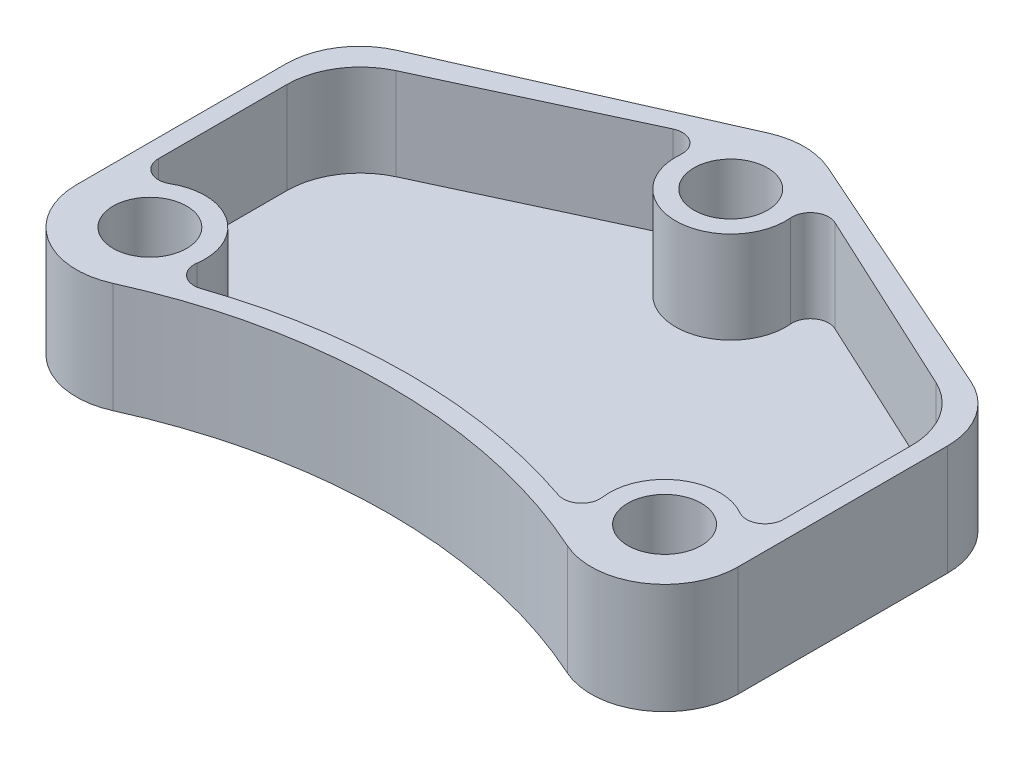
ISO-10303-21;
HEADER;
FILE_DESCRIPTION(('STEP AP214'),'2;1');
FILE_NAME('part.step','',(''),(''),'','','');
FILE_SCHEMA(('AUTOMOTIVE_DESIGN { 1 0 10303 214 1 1 1 1 }'));
ENDSEC;
DATA;
#1=APPLICATION_CONTEXT('core data for automotive mechanical design processes');
#2=APPLICATION_PROTOCOL_DEFINITION('international standard','automotive_design',2000,#1);
#3=PRODUCT_CONTEXT('',#1,'mechanical');
#4=PRODUCT('Part','Part','',(#3));
#5=PRODUCT_RELATED_PRODUCT_CATEGORY('part','',(#4));
#6=PRODUCT_DEFINITION_FORMATION('','',#4);
#7=PRODUCT_DEFINITION_CONTEXT('part definition',#1,'design');
#8=PRODUCT_DEFINITION('design','',#6,#7);
#9=PRODUCT_DEFINITION_SHAPE('','',#8);
#10=(LENGTH_UNIT() NAMED_UNIT(*) SI_UNIT(.MILLI.,.METRE.));
#11=(NAMED_UNIT(*) PLANE_ANGLE_UNIT() SI_UNIT($,.RADIAN.));
#12=(NAMED_UNIT(*) SI_UNIT($,.STERADIAN.) SOLID_ANGLE_UNIT());
#13=UNCERTAINTY_MEASURE_WITH_UNIT(LENGTH_MEASURE(1.E-05),#10,'distance_accuracy_value','');
#14=(GEOMETRIC_REPRESENTATION_CONTEXT(3) GLOBAL_UNCERTAINTY_ASSIGNED_CONTEXT((#13)) GLOBAL_UNIT_ASSIGNED_CONTEXT((#10,
#11,#12)) REPRESENTATION_CONTEXT('',''));
#15=CARTESIAN_POINT('',(0.,0.,0.));
#16=DIRECTION('',(0.,0.,1.));
#17=DIRECTION('',(1.,0.,0.));
#18=AXIS2_PLACEMENT_3D('',#15,#16,#17);
#19=CARTESIAN_POINT('',(70.,30.,88.0000000000001));
#20=DIRECTION('',(0.,-1.,0.));
#21=DIRECTION('',(0.,0.,-1.));
#22=AXIS2_PLACEMENT_3D('',#19,#20,#21);
#23=CYLINDRICAL_SURFACE('',#22,15.);
#24=DIRECTION('',(0.,-1.,0.));
#25=VECTOR('',#24,1.);
#26=CARTESIAN_POINT('',(77.5,30.,75.0096189432336));
#27=LINE('',#26,#25);
#28=CARTESIAN_POINT('',(77.5,30.,75.0096189432336));
#29=VERTEX_POINT('',#28);
#30=CARTESIAN_POINT('',(77.5,5.,75.0096189432336));
#31=VERTEX_POINT('',#30);
#32=EDGE_CURVE('E62',#29,#31,#27,.T.);
#33=ORIENTED_EDGE('',*,*,#32,.T.);
#34=CARTESIAN_POINT('',(70.,5.,88.0000000000001));
#35=DIRECTION('',(0.,-1.,0.));
#36=DIRECTION('',(0.,0.,-1.));
#37=AXIS2_PLACEMENT_3D('',#34,#35,#36);
#38=CIRCLE('',#37,15.);
#39=CARTESIAN_POINT('',(55.1442718779015,5.,90.0754136846162));
#40=VERTEX_POINT('',#39);
#41=EDGE_CURVE('E57',#31,#40,#38,.F.);
#42=ORIENTED_EDGE('',*,*,#41,.T.);
#43=DIRECTION('',(0.,-1.,0.));
#44=VECTOR('',#43,1.);
#45=CARTESIAN_POINT('',(55.1442718779015,30.,90.0754136846162));
#46=LINE('',#45,#44);
#47=CARTESIAN_POINT('',(55.1442718779015,30.,90.0754136846162));
#48=VERTEX_POINT('',#47);
#49=EDGE_CURVE('E47',#48,#40,#46,.T.);
#50=ORIENTED_EDGE('',*,*,#49,.F.);
#51=CARTESIAN_POINT('',(70.,30.,88.0000000000001));
#52=DIRECTION('',(0.,1.,0.));
#53=DIRECTION('',(0.,0.,1.));
#54=AXIS2_PLACEMENT_3D('',#51,#52,#53);
#55=CIRCLE('',#54,15.);
#56=EDGE_CURVE('E343',#48,#29,#55,.F.);
#57=ORIENTED_EDGE('',*,*,#56,.T.);
#58=EDGE_LOOP('',(#33,#42,#50,#57));
#59=FACE_BOUND('',#58,.T.);
#60=ADVANCED_FACE('F41',(#59),#23,.T.);
#61=CARTESIAN_POINT('',(50.1923625038687,30.,90.7672182461548));
#62=DIRECTION('',(0.,-1.,0.));
#63=DIRECTION('',(0.,0.,-1.));
#64=AXIS2_PLACEMENT_3D('',#61,#62,#63);
#65=CYLINDRICAL_SURFACE('',#64,4.99999999999999);
#66=CARTESIAN_POINT('',(50.1923625038687,5.,90.7672182461548));
#67=DIRECTION('',(0.,-1.,0.));
#68=DIRECTION('',(0.,0.,-1.));
#69=AXIS2_PLACEMENT_3D('',#66,#67,#68);
#70=CIRCLE('',#69,4.99999999999999);
#71=CARTESIAN_POINT('',(48.5732540360019,5.,95.497808882564));
#72=VERTEX_POINT('',#71);
#73=EDGE_CURVE('E378',#72,#40,#70,.F.);
#74=ORIENTED_EDGE('',*,*,#73,.F.);
#75=DIRECTION('',(0.,-1.,0.));
#76=VECTOR('',#75,1.);
#77=CARTESIAN_POINT('',(48.5732540360019,30.,95.497808882564));
#78=LINE('',#77,#76);
#79=CARTESIAN_POINT('',(48.5732540360019,30.,95.497808882564));
#80=VERTEX_POINT('',#79);
#81=EDGE_CURVE('E247',#80,#72,#78,.T.);
#82=ORIENTED_EDGE('',*,*,#81,.F.);
#83=CARTESIAN_POINT('',(50.1923625038687,30.,90.7672182461548));
#84=DIRECTION('',(0.,1.,0.));
#85=DIRECTION('',(0.,0.,1.));
#86=AXIS2_PLACEMENT_3D('',#83,#84,#85);
#87=CIRCLE('',#86,4.99999999999999);
#88=EDGE_CURVE('E345',#48,#80,#87,.F.);
#89=ORIENTED_EDGE('',*,*,#88,.F.);
#90=ORIENTED_EDGE('',*,*,#49,.T.);
#91=EDGE_LOOP('',(#74,#82,#89,#90));
#92=FACE_BOUND('',#91,.T.);
#93=ADVANCED_FACE('F428',(#92),#65,.F.);
#94=CARTESIAN_POINT('',(0.,30.,237.415527974839));
#95=DIRECTION('',(0.,-1.,0.));
#96=DIRECTION('',(0.,0.,-1.));
#97=AXIS2_PLACEMENT_3D('',#94,#95,#96);
#98=CYLINDRICAL_SURFACE('',#97,150.);
#99=ORIENTED_EDGE('',*,*,#81,.T.);
#100=CARTESIAN_POINT('',(0.,5.,237.415527974839));
#101=DIRECTION('',(0.,-1.,0.));
#102=DIRECTION('',(0.,0.,-1.));
#103=AXIS2_PLACEMENT_3D('',#100,#101,#102);
#104=CIRCLE('',#103,150.);
#105=CARTESIAN_POINT('',(-48.573254036002,5.,95.497808882564));
#106=VERTEX_POINT('',#105);
#107=EDGE_CURVE('E379',#72,#106,#104,.F.);
#108=ORIENTED_EDGE('',*,*,#107,.T.);
#109=DIRECTION('',(0.,-1.,0.));
#110=VECTOR('',#109,1.);
#111=CARTESIAN_POINT('',(-48.573254036002,30.,95.497808882564));
#112=LINE('',#111,#110);
#113=CARTESIAN_POINT('',(-48.573254036002,30.,95.497808882564));
#114=VERTEX_POINT('',#113);
#115=EDGE_CURVE('E244',#114,#106,#112,.T.);
#116=ORIENTED_EDGE('',*,*,#115,.F.);
#117=CARTESIAN_POINT('',(0.,30.,237.415527974839));
#118=DIRECTION('',(0.,1.,0.));
#119=DIRECTION('',(0.,0.,1.));
#120=AXIS2_PLACEMENT_3D('',#117,#118,#119);
#121=CIRCLE('',#120,150.);
#122=EDGE_CURVE('E338',#114,#80,#121,.F.);
#123=ORIENTED_EDGE('',*,*,#122,.T.);
#124=EDGE_LOOP('',(#99,#108,#116,#123));
#125=FACE_BOUND('',#124,.T.);
#126=ADVANCED_FACE('F431',(#125),#98,.T.);
#127=CARTESIAN_POINT('',(-50.1923625038687,30.,90.7672182461548));
#128=DIRECTION('',(0.,-1.,0.));
#129=DIRECTION('',(0.,0.,-1.));
#130=AXIS2_PLACEMENT_3D('',#127,#128,#129);
#131=CYLINDRICAL_SURFACE('',#130,4.99999999999999);
#132=ORIENTED_EDGE('',*,*,#115,.T.);
#133=CARTESIAN_POINT('',(-50.1923625038687,5.,90.7672182461548));
#134=DIRECTION('',(0.,-1.,0.));
#135=DIRECTION('',(0.,0.,-1.));
#136=AXIS2_PLACEMENT_3D('',#133,#134,#135);
#137=CIRCLE('',#136,4.99999999999999);
#138=CARTESIAN_POINT('',(-55.1442718779016,5.,90.0754136846162));
#139=VERTEX_POINT('',#138);
#140=EDGE_CURVE('E382',#106,#139,#137,.T.);
#141=ORIENTED_EDGE('',*,*,#140,.T.);
#142=DIRECTION('',(0.,-1.,0.));
#143=VECTOR('',#142,1.);
#144=CARTESIAN_POINT('',(-55.1442718779016,30.,90.0754136846162));
#145=LINE('',#144,#143);
#146=CARTESIAN_POINT('',(-55.1442718779016,30.,90.0754136846162));
#147=VERTEX_POINT('',#146);
#148=EDGE_CURVE('E245',#147,#139,#145,.T.);
#149=ORIENTED_EDGE('',*,*,#148,.F.);
#150=CARTESIAN_POINT('',(-50.1923625038687,30.,90.7672182461548));
#151=DIRECTION('',(0.,1.,0.));
#152=DIRECTION('',(0.,0.,1.));
#153=AXIS2_PLACEMENT_3D('',#150,#151,#152);
#154=CIRCLE('',#153,4.99999999999999);
#155=EDGE_CURVE('E336',#147,#114,#154,.T.);
#156=ORIENTED_EDGE('',*,*,#155,.T.);
#157=EDGE_LOOP('',(#132,#141,#149,#156));
#158=FACE_BOUND('',#157,.T.);
#159=ADVANCED_FACE('F432',(#158),#131,.F.);
#160=CARTESIAN_POINT('',(-70.,30.,88.0000000000001));
#161=DIRECTION('',(0.,-1.,0.));
#162=DIRECTION('',(0.,0.,-1.));
#163=AXIS2_PLACEMENT_3D('',#160,#161,#162);
#164=CYLINDRICAL_SURFACE('',#163,15.);
#165=CARTESIAN_POINT('',(-70.,5.,88.0000000000001));
#166=DIRECTION('',(0.,-1.,0.));
#167=DIRECTION('',(0.,0.,-1.));
#168=AXIS2_PLACEMENT_3D('',#165,#166,#167);
#169=CIRCLE('',#168,15.);
#170=CARTESIAN_POINT('',(-77.5,5.,75.0096189432336));
#171=VERTEX_POINT('',#170);
#172=EDGE_CURVE('E387',#171,#139,#169,.T.);
#173=ORIENTED_EDGE('',*,*,#172,.F.);
#174=DIRECTION('',(0.,-1.,0.));
#175=VECTOR('',#174,1.);
#176=CARTESIAN_POINT('',(-77.5000000000001,30.,75.0096189432335));
#177=LINE('',#176,#175);
#178=CARTESIAN_POINT('',(-77.5000000000001,30.,75.0096189432335));
#179=VERTEX_POINT('',#178);
#180=EDGE_CURVE('E239',#179,#171,#177,.T.);
#181=ORIENTED_EDGE('',*,*,#180,.F.);
#182=CARTESIAN_POINT('',(-70.,30.,88.0000000000001));
#183=DIRECTION('',(0.,1.,0.));
#184=DIRECTION('',(0.,0.,1.));
#185=AXIS2_PLACEMENT_3D('',#182,#183,#184);
#186=CIRCLE('',#185,15.);
#187=EDGE_CURVE('E334',#147,#179,#186,.T.);
#188=ORIENTED_EDGE('',*,*,#187,.F.);
#189=ORIENTED_EDGE('',*,*,#148,.T.);
#190=EDGE_LOOP('',(#173,#181,#188,#189));
#191=FACE_BOUND('',#190,.T.);
#192=ADVANCED_FACE('F445',(#191),#164,.T.);
#193=CARTESIAN_POINT('',(-80.0000000000001,30.,70.6794919243114));
#194=DIRECTION('',(0.,-1.,0.));
#195=DIRECTION('',(0.,0.,-1.));
#196=AXIS2_PLACEMENT_3D('',#193,#194,#195);
#197=CYLINDRICAL_SURFACE('',#196,5.00000000000001);
#198=CARTESIAN_POINT('',(-80.0000000000001,5.,70.6794919243114));
#199=DIRECTION('',(0.,-1.,0.));
#200=DIRECTION('',(0.,0.,-1.));
#201=AXIS2_PLACEMENT_3D('',#198,#199,#200);
#202=CIRCLE('',#201,5.00000000000001);
#203=CARTESIAN_POINT('',(-85.0000000000001,5.,70.6794919243114));
#204=VERTEX_POINT('',#203);
#205=EDGE_CURVE('E386',#204,#171,#202,.F.);
#206=ORIENTED_EDGE('',*,*,#205,.F.);
#207=DIRECTION('',(0.,-1.,0.));
#208=VECTOR('',#207,1.);
#209=CARTESIAN_POINT('',(-85.0000000000001,30.,70.6794919243114));
#210=LINE('',#209,#208);
#211=CARTESIAN_POINT('',(-85.0000000000001,30.,70.6794919243114));
#212=VERTEX_POINT('',#211);
#213=EDGE_CURVE('E237',#212,#204,#210,.T.);
#214=ORIENTED_EDGE('',*,*,#213,.F.);
#215=CARTESIAN_POINT('',(-80.0000000000001,30.,70.6794919243114));
#216=DIRECTION('',(0.,1.,0.));
#217=DIRECTION('',(0.,0.,1.));
#218=AXIS2_PLACEMENT_3D('',#215,#216,#217);
#219=CIRCLE('',#218,5.00000000000001);
#220=EDGE_CURVE('E332',#179,#212,#219,.F.);
#221=ORIENTED_EDGE('',*,*,#220,.F.);
#222=ORIENTED_EDGE('',*,*,#180,.T.);
#223=EDGE_LOOP('',(#206,#214,#221,#222));
#224=FACE_BOUND('',#223,.T.);
#225=ADVANCED_FACE('F447',(#224),#197,.F.);
#226=CARTESIAN_POINT('',(-85.,30.,0.));
#227=DIRECTION('',(1.,0.,0.));
#228=DIRECTION('',(0.,0.,-1.));
#229=AXIS2_PLACEMENT_3D('',#226,#227,#228);
#230=PLANE('',#229);
#231=ORIENTED_EDGE('',*,*,#213,.T.);
#232=DIRECTION('',(0.,0.,-1.));
#233=VECTOR('',#232,1.);
#234=CARTESIAN_POINT('',(-85.,5.,0.));
#235=LINE('',#234,#233);
#236=CARTESIAN_POINT('',(-85.0000000000001,5.,35.7709926715189));
#237=VERTEX_POINT('',#236);
#238=EDGE_CURVE('E395',#204,#237,#235,.T.);
#239=ORIENTED_EDGE('',*,*,#238,.T.);
#240=DIRECTION('',(0.,-1.,0.));
#241=VECTOR('',#240,1.);
#242=CARTESIAN_POINT('',(-85.0000000000001,30.,35.7709926715189));
#243=LINE('',#242,#241);
#244=CARTESIAN_POINT('',(-85.0000000000001,30.,35.7709926715189));
#245=VERTEX_POINT('',#244);
#246=EDGE_CURVE('E232',#245,#237,#243,.T.);
#247=ORIENTED_EDGE('',*,*,#246,.F.);
#248=DIRECTION('',(0.,0.,1.));
#249=VECTOR('',#248,1.);
#250=CARTESIAN_POINT('',(-85.,30.,0.));
#251=LINE('',#250,#249);
#252=EDGE_CURVE('E327',#245,#212,#251,.T.);
#253=ORIENTED_EDGE('',*,*,#252,.T.);
#254=EDGE_LOOP('',(#231,#239,#247,#253));
#255=FACE_BOUND('',#254,.T.);
#256=ADVANCED_FACE('F451',(#255),#230,.T.);
#257=CARTESIAN_POINT('',(-65.0000000000001,30.,35.7709926715189));
#258=DIRECTION('',(0.,-1.,0.));
#259=DIRECTION('',(0.,0.,-1.));
#260=AXIS2_PLACEMENT_3D('',#257,#258,#259);
#261=CYLINDRICAL_SURFACE('',#260,20.);
#262=ORIENTED_EDGE('',*,*,#246,.T.);
#263=CARTESIAN_POINT('',(-65.0000000000001,5.,35.7709926715189));
#264=DIRECTION('',(0.,-1.,0.));
#265=DIRECTION('',(0.,0.,-1.));
#266=AXIS2_PLACEMENT_3D('',#263,#264,#265);
#267=CIRCLE('',#266,20.);
#268=CARTESIAN_POINT('',(-73.4399590477228,5.,17.639056997886));
#269=VERTEX_POINT('',#268);
#270=EDGE_CURVE('E394',#237,#269,#267,.T.);
#271=ORIENTED_EDGE('',*,*,#270,.T.);
#272=DIRECTION('',(0.,-1.,0.));
#273=VECTOR('',#272,1.);
#274=CARTESIAN_POINT('',(-73.4399590477228,30.,17.639056997886));
#275=LINE('',#274,#273);
#276=CARTESIAN_POINT('',(-73.4399590477228,30.,17.639056997886));
#277=VERTEX_POINT('',#276);
#278=EDGE_CURVE('E229',#277,#269,#275,.T.);
#279=ORIENTED_EDGE('',*,*,#278,.F.);
#280=CARTESIAN_POINT('',(-65.0000000000001,30.,35.7709926715189));
#281=DIRECTION('',(0.,1.,0.));
#282=DIRECTION('',(0.,0.,1.));
#283=AXIS2_PLACEMENT_3D('',#280,#281,#282);
#284=CIRCLE('',#283,20.);
#285=EDGE_CURVE('E324',#277,#245,#284,.T.);
#286=ORIENTED_EDGE('',*,*,#285,.T.);
#287=EDGE_LOOP('',(#262,#271,#279,#286));
#288=FACE_BOUND('',#287,.T.);
#289=ADVANCED_FACE('F454',(#288),#261,.F.);
#290=CARTESIAN_POINT('',(-6.32996928579205,30.,-13.5989517552247));
#291=DIRECTION('',(-0.421997952386136,0.,-0.906596783681648));
#292=DIRECTION('',(-0.906596783681648,0.,0.421997952386136));
#293=AXIS2_PLACEMENT_3D('',#290,#291,#292);
#294=PLANE('',#293);
#295=DIRECTION('',(-0.906596783681648,0.,0.421997952386136));
#296=VECTOR('',#295,1.);
#297=CARTESIAN_POINT('',(-6.32996928579205,5.,-13.5989517552247));
#298=LINE('',#297,#296);
#299=CARTESIAN_POINT('',(-22.0326861989435,5.,-6.28973281299653));
#300=VERTEX_POINT('',#299);
#301=EDGE_CURVE('E397',#300,#269,#298,.T.);
#302=ORIENTED_EDGE('',*,*,#301,.F.);
#303=DIRECTION('',(0.,-1.,0.));
#304=VECTOR('',#303,1.);
#305=CARTESIAN_POINT('',(-22.0326861989435,30.,-6.28973281299653));
#306=LINE('',#305,#304);
#307=CARTESIAN_POINT('',(-22.0326861989435,30.,-6.28973281299653));
#308=VERTEX_POINT('',#307);
#309=EDGE_CURVE('E230',#308,#300,#306,.T.);
#310=ORIENTED_EDGE('',*,*,#309,.F.);
#311=DIRECTION('',(0.906596783681648,0.,-0.421997952386136));
#312=VECTOR('',#311,1.);
#313=CARTESIAN_POINT('',(-6.32996928579205,30.,-13.5989517552247));
#314=LINE('',#313,#312);
#315=EDGE_CURVE('E325',#277,#308,#314,.T.);
#316=ORIENTED_EDGE('',*,*,#315,.F.);
#317=ORIENTED_EDGE('',*,*,#278,.T.);
#318=EDGE_LOOP('',(#302,#310,#316,#317));
#319=FACE_BOUND('',#318,.T.);
#320=ADVANCED_FACE('F722',(#319),#294,.F.);
#321=CARTESIAN_POINT('',(-19.9226964370129,30.,-1.75674889458829));
#322=DIRECTION('',(0.,-1.,0.));
#323=DIRECTION('',(0.,0.,-1.));
#324=AXIS2_PLACEMENT_3D('',#321,#322,#323);
#325=CYLINDRICAL_SURFACE('',#324,5.);
#326=CARTESIAN_POINT('',(-19.9226964370129,5.,-1.75674889458829));
#327=DIRECTION('',(0.,-1.,0.));
#328=DIRECTION('',(0.,0.,-1.));
#329=AXIS2_PLACEMENT_3D('',#326,#327,#328);
#330=CIRCLE('',#329,5.);
#331=CARTESIAN_POINT('',(-14.9420223277596,5.,-1.31756167094121));
#332=VERTEX_POINT('',#331);
#333=EDGE_CURVE('E402',#332,#300,#330,.F.);
#334=ORIENTED_EDGE('',*,*,#333,.F.);
#335=DIRECTION('',(0.,-1.,0.));
#336=VECTOR('',#335,1.);
#337=CARTESIAN_POINT('',(-14.9420223277596,30.,-1.31756167094121));
#338=LINE('',#337,#336);
#339=CARTESIAN_POINT('',(-14.9420223277596,30.,-1.31756167094121));
#340=VERTEX_POINT('',#339);
#341=EDGE_CURVE('E221',#340,#332,#338,.T.);
#342=ORIENTED_EDGE('',*,*,#341,.F.);
#343=CARTESIAN_POINT('',(-19.9226964370129,30.,-1.75674889458829));
#344=DIRECTION('',(0.,1.,0.));
#345=DIRECTION('',(0.,0.,1.));
#346=AXIS2_PLACEMENT_3D('',#343,#344,#345);
#347=CIRCLE('',#346,5.);
#348=EDGE_CURVE('E317',#308,#340,#347,.F.);
#349=ORIENTED_EDGE('',*,*,#348,.F.);
#350=ORIENTED_EDGE('',*,*,#309,.T.);
#351=EDGE_LOOP('',(#334,#342,#349,#350));
#352=FACE_BOUND('',#351,.T.);
#353=ADVANCED_FACE('F713',(#352),#325,.F.);
#354=CARTESIAN_POINT('',(0.,30.,0.));
#355=DIRECTION('',(0.,-1.,0.));
#356=DIRECTION('',(0.,0.,-1.));
#357=AXIS2_PLACEMENT_3D('',#354,#355,#356);
#358=CYLINDRICAL_SURFACE('',#357,15.);
#359=CARTESIAN_POINT('',(0.,5.,0.));
#360=DIRECTION('',(0.,-1.,0.));
#361=DIRECTION('',(0.,0.,-1.));
#362=AXIS2_PLACEMENT_3D('',#359,#360,#361);
#363=CIRCLE('',#362,15.);
#364=CARTESIAN_POINT('',(14.9420223277597,5.,-1.31756167094122));
#365=VERTEX_POINT('',#364);
#366=EDGE_CURVE('E404',#365,#332,#363,.T.);
#367=ORIENTED_EDGE('',*,*,#366,.F.);
#368=DIRECTION('',(0.,-1.,0.));
#369=VECTOR('',#368,1.);
#370=CARTESIAN_POINT('',(14.9420223277597,30.,-1.31756167094122));
#371=LINE('',#370,#369);
#372=CARTESIAN_POINT('',(14.9420223277597,30.,-1.31756167094122));
#373=VERTEX_POINT('',#372);
#374=EDGE_CURVE('E222',#373,#365,#371,.T.);
#375=ORIENTED_EDGE('',*,*,#374,.F.);
#376=CARTESIAN_POINT('',(0.,30.,0.));
#377=DIRECTION('',(0.,1.,0.));
#378=DIRECTION('',(0.,0.,1.));
#379=AXIS2_PLACEMENT_3D('',#376,#377,#378);
#380=CIRCLE('',#379,15.);
#381=EDGE_CURVE('E320',#340,#373,#380,.T.);
#382=ORIENTED_EDGE('',*,*,#381,.F.);
#383=ORIENTED_EDGE('',*,*,#341,.T.);
#384=EDGE_LOOP('',(#367,#375,#382,#383));
#385=FACE_BOUND('',#384,.T.);
#386=ADVANCED_FACE('F487',(#385),#358,.T.);
#387=CARTESIAN_POINT('',(19.9226964370129,30.,-1.75674889458829));
#388=DIRECTION('',(0.,-1.,0.));
#389=DIRECTION('',(0.,0.,-1.));
#390=AXIS2_PLACEMENT_3D('',#387,#388,#389);
#391=CYLINDRICAL_SURFACE('',#390,5.);
#392=ORIENTED_EDGE('',*,*,#374,.T.);
#393=CARTESIAN_POINT('',(19.9226964370129,5.,-1.75674889458829));
#394=DIRECTION('',(0.,-1.,0.));
#395=DIRECTION('',(0.,0.,-1.));
#396=AXIS2_PLACEMENT_3D('',#393,#394,#395);
#397=CIRCLE('',#396,5.);
#398=CARTESIAN_POINT('',(22.0326861989435,5.,-6.28973281299653));
#399=VERTEX_POINT('',#398);
#400=EDGE_CURVE('E410',#365,#399,#397,.T.);
#401=ORIENTED_EDGE('',*,*,#400,.T.);
#402=DIRECTION('',(0.,-1.,0.));
#403=VECTOR('',#402,1.);
#404=CARTESIAN_POINT('',(22.0326861989435,30.,-6.28973281299653));
#405=LINE('',#404,#403);
#406=CARTESIAN_POINT('',(22.0326861989435,30.,-6.28973281299653));
#407=VERTEX_POINT('',#406);
#408=EDGE_CURVE('E212',#407,#399,#405,.T.);
#409=ORIENTED_EDGE('',*,*,#408,.F.);
#410=CARTESIAN_POINT('',(19.9226964370129,30.,-1.75674889458829));
#411=DIRECTION('',(0.,1.,0.));
#412=DIRECTION('',(0.,0.,1.));
#413=AXIS2_PLACEMENT_3D('',#410,#411,#412);
#414=CIRCLE('',#413,5.);
#415=EDGE_CURVE('E314',#407,#373,#414,.T.);
#416=ORIENTED_EDGE('',*,*,#415,.T.);
#417=EDGE_LOOP('',(#392,#401,#409,#416));
#418=FACE_BOUND('',#417,.T.);
#419=ADVANCED_FACE('F479',(#418),#391,.F.);
#420=CARTESIAN_POINT('',(6.32996928579205,30.,-13.5989517552247));
#421=DIRECTION('',(-0.421997952386136,0.,0.906596783681648));
#422=DIRECTION('',(0.906596783681648,0.,0.421997952386136));
#423=AXIS2_PLACEMENT_3D('',#420,#421,#422);
#424=PLANE('',#423);
#425=ORIENTED_EDGE('',*,*,#408,.T.);
#426=DIRECTION('',(0.906596783681648,0.,0.421997952386136));
#427=VECTOR('',#426,1.);
#428=CARTESIAN_POINT('',(6.32996928579205,5.,-13.5989517552247));
#429=LINE('',#428,#427);
#430=CARTESIAN_POINT('',(73.4399590477228,5.,17.639056997886));
#431=VERTEX_POINT('',#430);
#432=EDGE_CURVE('E409',#399,#431,#429,.T.);
#433=ORIENTED_EDGE('',*,*,#432,.T.);
#434=DIRECTION('',(0.,-1.,0.));
#435=VECTOR('',#434,1.);
#436=CARTESIAN_POINT('',(73.4399590477228,30.,17.639056997886));
#437=LINE('',#436,#435);
#438=CARTESIAN_POINT('',(73.4399590477228,30.,17.639056997886));
#439=VERTEX_POINT('',#438);
#440=EDGE_CURVE('E215',#439,#431,#437,.T.);
#441=ORIENTED_EDGE('',*,*,#440,.F.);
#442=DIRECTION('',(-0.906596783681648,0.,-0.421997952386136));
#443=VECTOR('',#442,1.);
#444=CARTESIAN_POINT('',(6.32996928579205,30.,-13.5989517552247));
#445=LINE('',#444,#443);
#446=EDGE_CURVE('E204',#439,#407,#445,.T.);
#447=ORIENTED_EDGE('',*,*,#446,.T.);
#448=EDGE_LOOP('',(#425,#433,#441,#447));
#449=FACE_BOUND('',#448,.T.);
#450=ADVANCED_FACE('F481',(#449),#424,.T.);
#451=CARTESIAN_POINT('',(65.0000000000001,30.,35.7709926715189));
#452=DIRECTION('',(0.,-1.,0.));
#453=DIRECTION('',(0.,0.,-1.));
#454=AXIS2_PLACEMENT_3D('',#451,#452,#453);
#455=CYLINDRICAL_SURFACE('',#454,20.);
#456=CARTESIAN_POINT('',(65.0000000000001,5.,35.7709926715189));
#457=DIRECTION('',(0.,-1.,0.));
#458=DIRECTION('',(0.,0.,-1.));
#459=AXIS2_PLACEMENT_3D('',#456,#457,#458);
#460=CIRCLE('',#459,20.);
#461=CARTESIAN_POINT('',(85.0000000000001,5.,35.7709926715189));
#462=VERTEX_POINT('',#461);
#463=EDGE_CURVE('E211',#462,#431,#460,.F.);
#464=ORIENTED_EDGE('',*,*,#463,.F.);
#465=DIRECTION('',(0.,-1.,0.));
#466=VECTOR('',#465,1.);
#467=CARTESIAN_POINT('',(85.0000000000001,30.,35.7709926715189));
#468=LINE('',#467,#466);
#469=CARTESIAN_POINT('',(85.0000000000001,30.,35.7709926715189));
#470=VERTEX_POINT('',#469);
#471=EDGE_CURVE('E189',#470,#462,#468,.T.);
#472=ORIENTED_EDGE('',*,*,#471,.F.);
#473=CARTESIAN_POINT('',(65.0000000000001,30.,35.7709926715189));
#474=DIRECTION('',(0.,1.,0.));
#475=DIRECTION('',(0.,0.,1.));
#476=AXIS2_PLACEMENT_3D('',#473,#474,#475);
#477=CIRCLE('',#476,20.);
#478=EDGE_CURVE('E198',#439,#470,#477,.F.);
#479=ORIENTED_EDGE('',*,*,#478,.F.);
#480=ORIENTED_EDGE('',*,*,#440,.T.);
#481=EDGE_LOOP('',(#464,#472,#479,#480));
#482=FACE_BOUND('',#481,.T.);
#483=ADVANCED_FACE('F207',(#482),#455,.F.);
#484=CARTESIAN_POINT('',(85.,30.,0.));
#485=DIRECTION('',(1.,0.,0.));
#486=DIRECTION('',(0.,0.,-1.));
#487=AXIS2_PLACEMENT_3D('',#484,#485,#486);
#488=PLANE('',#487);
#489=DIRECTION('',(0.,0.,-1.));
#490=VECTOR('',#489,1.);
#491=CARTESIAN_POINT('',(85.,5.,0.));
#492=LINE('',#491,#490);
#493=CARTESIAN_POINT('',(85.0000000000001,5.,70.6794919243114));
#494=VERTEX_POINT('',#493);
#495=EDGE_CURVE('E413',#494,#462,#492,.T.);
#496=ORIENTED_EDGE('',*,*,#495,.F.);
#497=DIRECTION('',(0.,-1.,0.));
#498=VECTOR('',#497,1.);
#499=CARTESIAN_POINT('',(85.0000000000001,30.,70.6794919243114));
#500=LINE('',#499,#498);
#501=CARTESIAN_POINT('',(85.0000000000001,30.,70.6794919243114));
#502=VERTEX_POINT('',#501);
#503=EDGE_CURVE('E195',#502,#494,#500,.T.);
#504=ORIENTED_EDGE('',*,*,#503,.F.);
#505=DIRECTION('',(0.,0.,1.));
#506=VECTOR('',#505,1.);
#507=CARTESIAN_POINT('',(85.,30.,0.));
#508=LINE('',#507,#506);
#509=EDGE_CURVE('E184',#470,#502,#508,.T.);
#510=ORIENTED_EDGE('',*,*,#509,.F.);
#511=ORIENTED_EDGE('',*,*,#471,.T.);
#512=EDGE_LOOP('',(#496,#504,#510,#511));
#513=FACE_BOUND('',#512,.T.);
#514=ADVANCED_FACE('F190',(#513),#488,.F.);
#515=CARTESIAN_POINT('',(80.0000000000001,30.,70.6794919243114));
#516=DIRECTION('',(0.,-1.,0.));
#517=DIRECTION('',(0.,0.,-1.));
#518=AXIS2_PLACEMENT_3D('',#515,#516,#517);
#519=CYLINDRICAL_SURFACE('',#518,5.00000000000001);
#520=ORIENTED_EDGE('',*,*,#503,.T.);
#521=CARTESIAN_POINT('',(80.0000000000001,5.,70.6794919243114));
#522=DIRECTION('',(0.,-1.,0.));
#523=DIRECTION('',(0.,0.,-1.));
#524=AXIS2_PLACEMENT_3D('',#521,#522,#523);
#525=CIRCLE('',#524,5.00000000000001);
#526=EDGE_CURVE('E11',#494,#31,#525,.T.);
#527=ORIENTED_EDGE('',*,*,#526,.T.);
#528=ORIENTED_EDGE('',*,*,#32,.F.);
#529=CARTESIAN_POINT('',(80.0000000000001,30.,70.6794919243114));
#530=DIRECTION('',(0.,1.,0.));
#531=DIRECTION('',(0.,0.,1.));
#532=AXIS2_PLACEMENT_3D('',#529,#530,#531);
#533=CIRCLE('',#532,5.00000000000001);
#534=EDGE_CURVE('E194',#29,#502,#533,.T.);
#535=ORIENTED_EDGE('',*,*,#534,.T.);
#536=EDGE_LOOP('',(#520,#527,#528,#535));
#537=FACE_BOUND('',#536,.T.);
#538=ADVANCED_FACE('F425',(#537),#519,.F.);
#539=CARTESIAN_POINT('',(-70.,30.,88.0000000000001));
#540=DIRECTION('',(0.,-1.,0.));
#541=DIRECTION('',(0.,0.,-1.));
#542=AXIS2_PLACEMENT_3D('',#539,#540,#541);
#543=CYLINDRICAL_SURFACE('',#542,20.);
#544=CARTESIAN_POINT('',(-70.,0.,88.0000000000001));
#545=DIRECTION('',(0.,1.,0.));
#546=DIRECTION('',(0.,0.,1.));
#547=AXIS2_PLACEMENT_3D('',#544,#545,#546);
#548=CIRCLE('',#547,20.);
#549=CARTESIAN_POINT('',(-90.,0.,88.0000000000002));
#550=VERTEX_POINT('',#549);
#551=CARTESIAN_POINT('',(-61.764705882353,0.,106.225803982153));
#552=VERTEX_POINT('',#551);
#553=EDGE_CURVE('E309',#550,#552,#548,.T.);
#554=ORIENTED_EDGE('',*,*,#553,.T.);
#555=DIRECTION('',(0.,-1.,0.));
#556=VECTOR('',#555,1.);
#557=CARTESIAN_POINT('',(-61.764705882353,30.,106.225803982153));
#558=LINE('',#557,#556);
#559=CARTESIAN_POINT('',(-61.764705882353,30.,106.225803982153));
#560=VERTEX_POINT('',#559);
#561=EDGE_CURVE('E267',#560,#552,#558,.T.);
#562=ORIENTED_EDGE('',*,*,#561,.F.);
#563=CARTESIAN_POINT('',(-70.,30.,88.0000000000001));
#564=DIRECTION('',(0.,1.,0.));
#565=DIRECTION('',(0.,0.,1.));
#566=AXIS2_PLACEMENT_3D('',#563,#564,#565);
#567=CIRCLE('',#566,20.);
#568=CARTESIAN_POINT('',(-90.,30.,88.0000000000002));
#569=VERTEX_POINT('',#568);
#570=EDGE_CURVE('E279',#569,#560,#567,.T.);
#571=ORIENTED_EDGE('',*,*,#570,.F.);
#572=DIRECTION('',(0.,-1.,0.));
#573=VECTOR('',#572,1.);
#574=CARTESIAN_POINT('',(-90.,30.,88.0000000000002));
#575=LINE('',#574,#573);
#576=EDGE_CURVE('E102',#569,#550,#575,.T.);
#577=ORIENTED_EDGE('',*,*,#576,.T.);
#578=EDGE_LOOP('',(#554,#562,#571,#577));
#579=FACE_BOUND('',#578,.T.);
#580=ADVANCED_FACE('F43',(#579),#543,.T.);
#581=CARTESIAN_POINT('',(0.,30.,242.919333848297));
#582=DIRECTION('',(0.,-1.,0.));
#583=DIRECTION('',(0.,0.,-1.));
#584=AXIS2_PLACEMENT_3D('',#581,#582,#583);
#585=CYLINDRICAL_SURFACE('',#584,150.);
#586=CARTESIAN_POINT('',(0.,0.,242.919333848297));
#587=DIRECTION('',(0.,1.,0.));
#588=DIRECTION('',(0.,0.,1.));
#589=AXIS2_PLACEMENT_3D('',#586,#587,#588);
#590=CIRCLE('',#589,150.);
#591=CARTESIAN_POINT('',(61.764705882353,0.,106.225803982153));
#592=VERTEX_POINT('',#591);
#593=EDGE_CURVE('E306',#552,#592,#590,.F.);
#594=ORIENTED_EDGE('',*,*,#593,.T.);
#595=DIRECTION('',(0.,-1.,0.));
#596=VECTOR('',#595,1.);
#597=CARTESIAN_POINT('',(61.764705882353,30.,106.225803982153));
#598=LINE('',#597,#596);
#599=CARTESIAN_POINT('',(61.764705882353,30.,106.225803982153));
#600=VERTEX_POINT('',#599);
#601=EDGE_CURVE('E268',#600,#592,#598,.T.);
#602=ORIENTED_EDGE('',*,*,#601,.F.);
#603=CARTESIAN_POINT('',(0.,30.,242.919333848297));
#604=DIRECTION('',(0.,1.,0.));
#605=DIRECTION('',(0.,0.,1.));
#606=AXIS2_PLACEMENT_3D('',#603,#604,#605);
#607=CIRCLE('',#606,150.);
#608=EDGE_CURVE('E115',#560,#600,#607,.F.);
#609=ORIENTED_EDGE('',*,*,#608,.F.);
#610=ORIENTED_EDGE('',*,*,#561,.T.);
#611=EDGE_LOOP('',(#594,#602,#609,#610));
#612=FACE_BOUND('',#611,.T.);
#613=ADVANCED_FACE('F545',(#612),#585,.F.);
#614=CARTESIAN_POINT('',(70.,30.,88.0000000000001));
#615=DIRECTION('',(0.,-1.,0.));
#616=DIRECTION('',(0.,0.,-1.));
#617=AXIS2_PLACEMENT_3D('',#614,#615,#616);
#618=CYLINDRICAL_SURFACE('',#617,20.);
#619=CARTESIAN_POINT('',(70.,0.,88.0000000000001));
#620=DIRECTION('',(0.,1.,0.));
#621=DIRECTION('',(0.,0.,1.));
#622=AXIS2_PLACEMENT_3D('',#619,#620,#621);
#623=CIRCLE('',#622,20.);
#624=CARTESIAN_POINT('',(90.,0.,88.0000000000002));
#625=VERTEX_POINT('',#624);
#626=EDGE_CURVE('E304',#625,#592,#623,.F.);
#627=ORIENTED_EDGE('',*,*,#626,.F.);
#628=DIRECTION('',(0.,-1.,0.));
#629=VECTOR('',#628,1.);
#630=CARTESIAN_POINT('',(90.,30.,88.0000000000002));
#631=LINE('',#630,#629);
#632=CARTESIAN_POINT('',(90.,30.,88.0000000000002));
#633=VERTEX_POINT('',#632);
#634=EDGE_CURVE('E266',#633,#625,#631,.T.);
#635=ORIENTED_EDGE('',*,*,#634,.F.);
#636=CARTESIAN_POINT('',(70.,30.,88.0000000000001));
#637=DIRECTION('',(0.,1.,0.));
#638=DIRECTION('',(0.,0.,1.));
#639=AXIS2_PLACEMENT_3D('',#636,#637,#638);
#640=CIRCLE('',#639,20.);
#641=EDGE_CURVE('E375',#633,#600,#640,.F.);
#642=ORIENTED_EDGE('',*,*,#641,.T.);
#643=ORIENTED_EDGE('',*,*,#601,.T.);
#644=EDGE_LOOP('',(#627,#635,#642,#643));
#645=FACE_BOUND('',#644,.T.);
#646=ADVANCED_FACE('F537',(#645),#618,.T.);
#647=CARTESIAN_POINT('',(89.9999999999999,30.,0.));
#648=DIRECTION('',(1.,0.,0.));
#649=DIRECTION('',(0.,0.,-1.));
#650=AXIS2_PLACEMENT_3D('',#647,#648,#649);
#651=PLANE('',#650);
#652=DIRECTION('',(0.,0.,1.));
#653=VECTOR('',#652,1.);
#654=CARTESIAN_POINT('',(89.9999999999999,0.,0.));
#655=LINE('',#654,#653);
#656=CARTESIAN_POINT('',(90.,0.,31.0139604920428));
#657=VERTEX_POINT('',#656);
#658=EDGE_CURVE('E305',#657,#625,#655,.T.);
#659=ORIENTED_EDGE('',*,*,#658,.F.);
#660=DIRECTION('',(0.,-1.,0.));
#661=VECTOR('',#660,1.);
#662=CARTESIAN_POINT('',(90.,30.,31.0139604920428));
#663=LINE('',#662,#661);
#664=CARTESIAN_POINT('',(90.,30.,31.0139604920428));
#665=VERTEX_POINT('',#664);
#666=EDGE_CURVE('E262',#665,#657,#663,.T.);
#667=ORIENTED_EDGE('',*,*,#666,.F.);
#668=DIRECTION('',(0.,0.,1.));
#669=VECTOR('',#668,1.);
#670=CARTESIAN_POINT('',(89.9999999999999,30.,0.));
#671=LINE('',#670,#669);
#672=EDGE_CURVE('E369',#665,#633,#671,.T.);
#673=ORIENTED_EDGE('',*,*,#672,.T.);
#674=ORIENTED_EDGE('',*,*,#634,.T.);
#675=EDGE_LOOP('',(#659,#667,#673,#674));
#676=FACE_BOUND('',#675,.T.);
#677=ADVANCED_FACE('F532',(#676),#651,.T.);
#678=CARTESIAN_POINT('',(70.,30.,31.0139604920429));
#679=DIRECTION('',(0.,-1.,0.));
#680=DIRECTION('',(0.,0.,-1.));
#681=AXIS2_PLACEMENT_3D('',#678,#679,#680);
#682=CYLINDRICAL_SURFACE('',#681,20.);
#683=CARTESIAN_POINT('',(70.,0.,31.0139604920429));
#684=DIRECTION('',(0.,1.,0.));
#685=DIRECTION('',(0.,0.,1.));
#686=AXIS2_PLACEMENT_3D('',#683,#684,#685);
#687=CIRCLE('',#686,20.);
#688=CARTESIAN_POINT('',(78.1015719105229,0.,12.7283231616509));
#689=VERTEX_POINT('',#688);
#690=EDGE_CURVE('E298',#657,#689,#687,.T.);
#691=ORIENTED_EDGE('',*,*,#690,.T.);
#692=DIRECTION('',(0.,-1.,0.));
#693=VECTOR('',#692,1.);
#694=CARTESIAN_POINT('',(78.1015719105229,30.,12.7283231616509));
#695=LINE('',#694,#693);
#696=CARTESIAN_POINT('',(78.1015719105229,30.,12.7283231616509));
#697=VERTEX_POINT('',#696);
#698=EDGE_CURVE('E265',#697,#689,#695,.T.);
#699=ORIENTED_EDGE('',*,*,#698,.F.);
#700=CARTESIAN_POINT('',(70.,30.,31.0139604920429));
#701=DIRECTION('',(0.,1.,0.));
#702=DIRECTION('',(0.,0.,1.));
#703=AXIS2_PLACEMENT_3D('',#700,#701,#702);
#704=CIRCLE('',#703,20.);
#705=EDGE_CURVE('E370',#665,#697,#704,.T.);
#706=ORIENTED_EDGE('',*,*,#705,.F.);
#707=ORIENTED_EDGE('',*,*,#666,.T.);
#708=EDGE_LOOP('',(#691,#699,#706,#707));
#709=FACE_BOUND('',#708,.T.);
#710=ADVANCED_FACE('F533',(#709),#682,.T.);
#711=CARTESIAN_POINT('',(8.10157191052293,30.,-18.2856373303921));
#712=DIRECTION('',(0.405078595526146,0.,-0.914281866519601));
#713=DIRECTION('',(-0.914281866519601,0.,-0.405078595526146));
#714=AXIS2_PLACEMENT_3D('',#711,#712,#713);
#715=PLANE('',#714);
#716=DIRECTION('',(0.914281866519601,0.,0.405078595526146));
#717=VECTOR('',#716,1.);
#718=CARTESIAN_POINT('',(8.10157191052293,0.,-18.2856373303921));
#719=LINE('',#718,#717);
#720=CARTESIAN_POINT('',(8.10157191052292,0.,-18.2856373303921));
#721=VERTEX_POINT('',#720);
#722=EDGE_CURVE('E296',#721,#689,#719,.T.);
#723=ORIENTED_EDGE('',*,*,#722,.F.);
#724=DIRECTION('',(0.,-1.,0.));
#725=VECTOR('',#724,1.);
#726=CARTESIAN_POINT('',(8.10157191052292,30.,-18.2856373303921));
#727=LINE('',#726,#725);
#728=CARTESIAN_POINT('',(8.10157191052292,30.,-18.2856373303921));
#729=VERTEX_POINT('',#728);
#730=EDGE_CURVE('E257',#729,#721,#727,.T.);
#731=ORIENTED_EDGE('',*,*,#730,.F.);
#732=DIRECTION('',(0.914281866519601,0.,0.405078595526146));
#733=VECTOR('',#732,1.);
#734=CARTESIAN_POINT('',(8.10157191052293,30.,-18.2856373303921));
#735=LINE('',#734,#733);
#736=EDGE_CURVE('E365',#729,#697,#735,.T.);
#737=ORIENTED_EDGE('',*,*,#736,.T.);
#738=ORIENTED_EDGE('',*,*,#698,.T.);
#739=EDGE_LOOP('',(#723,#731,#737,#738));
#740=FACE_BOUND('',#739,.T.);
#741=ADVANCED_FACE('F527',(#740),#715,.T.);
#742=CARTESIAN_POINT('',(0.,30.,0.));
#743=DIRECTION('',(0.,-1.,0.));
#744=DIRECTION('',(0.,0.,-1.));
#745=AXIS2_PLACEMENT_3D('',#742,#743,#744);
#746=CYLINDRICAL_SURFACE('',#745,20.);
#747=CARTESIAN_POINT('',(0.,0.,0.));
#748=DIRECTION('',(0.,1.,0.));
#749=DIRECTION('',(0.,0.,1.));
#750=AXIS2_PLACEMENT_3D('',#747,#748,#749);
#751=CIRCLE('',#750,20.);
#752=CARTESIAN_POINT('',(-8.10157191052289,0.,-18.285637330392));
#753=VERTEX_POINT('',#752);
#754=EDGE_CURVE('E291',#721,#753,#751,.T.);
#755=ORIENTED_EDGE('',*,*,#754,.T.);
#756=DIRECTION('',(0.,-1.,0.));
#757=VECTOR('',#756,1.);
#758=CARTESIAN_POINT('',(-8.10157191052289,30.,-18.285637330392));
#759=LINE('',#758,#757);
#760=CARTESIAN_POINT('',(-8.10157191052289,30.,-18.285637330392));
#761=VERTEX_POINT('',#760);
#762=EDGE_CURVE('E256',#761,#753,#759,.T.);
#763=ORIENTED_EDGE('',*,*,#762,.F.);
#764=CARTESIAN_POINT('',(0.,30.,0.));
#765=DIRECTION('',(0.,1.,0.));
#766=DIRECTION('',(0.,0.,1.));
#767=AXIS2_PLACEMENT_3D('',#764,#765,#766);
#768=CIRCLE('',#767,20.);
#769=EDGE_CURVE('E362',#729,#761,#768,.T.);
#770=ORIENTED_EDGE('',*,*,#769,.F.);
#771=ORIENTED_EDGE('',*,*,#730,.T.);
#772=EDGE_LOOP('',(#755,#763,#770,#771));
#773=FACE_BOUND('',#772,.T.);
#774=ADVANCED_FACE('F522',(#773),#746,.T.);
#775=CARTESIAN_POINT('',(-8.10157191052291,30.,-18.285637330392));
#776=DIRECTION('',(0.405078595526146,0.,0.914281866519601));
#777=DIRECTION('',(0.914281866519601,0.,-0.405078595526146));
#778=AXIS2_PLACEMENT_3D('',#775,#776,#777);
#779=PLANE('',#778);
#780=DIRECTION('',(-0.914281866519601,0.,0.405078595526146));
#781=VECTOR('',#780,1.);
#782=CARTESIAN_POINT('',(-8.10157191052291,0.,-18.285637330392));
#783=LINE('',#782,#781);
#784=CARTESIAN_POINT('',(-78.1015719105228,0.,12.7283231616509));
#785=VERTEX_POINT('',#784);
#786=EDGE_CURVE('E289',#753,#785,#783,.T.);
#787=ORIENTED_EDGE('',*,*,#786,.T.);
#788=DIRECTION('',(0.,-1.,0.));
#789=VECTOR('',#788,1.);
#790=CARTESIAN_POINT('',(-78.1015719105228,30.,12.7283231616509));
#791=LINE('',#790,#789);
#792=CARTESIAN_POINT('',(-78.1015719105228,30.,12.7283231616509));
#793=VERTEX_POINT('',#792);
#794=EDGE_CURVE('E258',#793,#785,#791,.T.);
#795=ORIENTED_EDGE('',*,*,#794,.F.);
#796=DIRECTION('',(-0.914281866519601,0.,0.405078595526146));
#797=VECTOR('',#796,1.);
#798=CARTESIAN_POINT('',(-8.10157191052291,30.,-18.285637330392));
#799=LINE('',#798,#797);
#800=EDGE_CURVE('E359',#761,#793,#799,.T.);
#801=ORIENTED_EDGE('',*,*,#800,.F.);
#802=ORIENTED_EDGE('',*,*,#762,.T.);
#803=EDGE_LOOP('',(#787,#795,#801,#802));
#804=FACE_BOUND('',#803,.T.);
#805=ADVANCED_FACE('F518',(#804),#779,.F.);
#806=CARTESIAN_POINT('',(-70.,30.,31.0139604920429));
#807=DIRECTION('',(0.,-1.,0.));
#808=DIRECTION('',(0.,0.,-1.));
#809=AXIS2_PLACEMENT_3D('',#806,#807,#808);
#810=CYLINDRICAL_SURFACE('',#809,20.);
#811=CARTESIAN_POINT('',(-70.,0.,31.0139604920429));
#812=DIRECTION('',(0.,1.,0.));
#813=DIRECTION('',(0.,0.,1.));
#814=AXIS2_PLACEMENT_3D('',#811,#812,#813);
#815=CIRCLE('',#814,20.);
#816=CARTESIAN_POINT('',(-90.,0.,31.0139604920429));
#817=VERTEX_POINT('',#816);
#818=EDGE_CURVE('E290',#817,#785,#815,.F.);
#819=ORIENTED_EDGE('',*,*,#818,.F.);
#820=DIRECTION('',(0.,-1.,0.));
#821=VECTOR('',#820,1.);
#822=CARTESIAN_POINT('',(-90.,30.,31.0139604920429));
#823=LINE('',#822,#821);
#824=CARTESIAN_POINT('',(-90.,30.,31.0139604920429));
#825=VERTEX_POINT('',#824);
#826=EDGE_CURVE('E255',#825,#817,#823,.T.);
#827=ORIENTED_EDGE('',*,*,#826,.F.);
#828=CARTESIAN_POINT('',(-70.,30.,31.0139604920429));
#829=DIRECTION('',(0.,1.,0.));
#830=DIRECTION('',(0.,0.,1.));
#831=AXIS2_PLACEMENT_3D('',#828,#829,#830);
#832=CIRCLE('',#831,20.);
#833=EDGE_CURVE('E360',#825,#793,#832,.F.);
#834=ORIENTED_EDGE('',*,*,#833,.T.);
#835=ORIENTED_EDGE('',*,*,#794,.T.);
#836=EDGE_LOOP('',(#819,#827,#834,#835));
#837=FACE_BOUND('',#836,.T.);
#838=ADVANCED_FACE('F503',(#837),#810,.T.);
#839=CARTESIAN_POINT('',(0.,30.,0.));
#840=DIRECTION('',(0.,-1.,0.));
#841=DIRECTION('',(0.,0.,-1.));
#842=AXIS2_PLACEMENT_3D('',#839,#840,#841);
#843=CYLINDRICAL_SURFACE('',#842,10.);
#844=CARTESIAN_POINT('',(0.,0.,0.));
#845=DIRECTION('',(0.,1.,0.));
#846=DIRECTION('',(0.,0.,1.));
#847=AXIS2_PLACEMENT_3D('',#844,#845,#846);
#848=CIRCLE('',#847,10.);
#849=CARTESIAN_POINT('',(0.,0.,10.));
#850=VERTEX_POINT('',#849);
#851=EDGE_CURVE('E274',#850,#850,#848,.T.);
#852=ORIENTED_EDGE('',*,*,#851,.F.);
#853=EDGE_LOOP('',(#852));
#854=FACE_BOUND('',#853,.T.);
#855=CARTESIAN_POINT('',(0.,30.,0.));
#856=DIRECTION('',(0.,1.,0.));
#857=DIRECTION('',(0.,0.,1.));
#858=AXIS2_PLACEMENT_3D('',#855,#856,#857);
#859=CIRCLE('',#858,10.);
#860=CARTESIAN_POINT('',(0.,30.,10.));
#861=VERTEX_POINT('',#860);
#862=EDGE_CURVE('E347',#861,#861,#859,.T.);
#863=ORIENTED_EDGE('',*,*,#862,.T.);
#864=EDGE_LOOP('',(#863));
#865=FACE_BOUND('',#864,.T.);
#866=ADVANCED_FACE('F498',(#854,#865),#843,.F.);
#867=CARTESIAN_POINT('',(-70.,30.,88.0000000000001));
#868=DIRECTION('',(0.,-1.,0.));
#869=DIRECTION('',(0.,0.,-1.));
#870=AXIS2_PLACEMENT_3D('',#867,#868,#869);
#871=CYLINDRICAL_SURFACE('',#870,10.);
#872=CARTESIAN_POINT('',(-70.,0.,88.0000000000001));
#873=DIRECTION('',(0.,1.,0.));
#874=DIRECTION('',(0.,0.,1.));
#875=AXIS2_PLACEMENT_3D('',#872,#873,#874);
#876=CIRCLE('',#875,10.);
#877=CARTESIAN_POINT('',(-70.,0.,98.0000000000001));
#878=VERTEX_POINT('',#877);
#879=EDGE_CURVE('E276',#878,#878,#876,.T.);
#880=ORIENTED_EDGE('',*,*,#879,.F.);
#881=EDGE_LOOP('',(#880));
#882=FACE_BOUND('',#881,.T.);
#883=CARTESIAN_POINT('',(-70.,30.,88.0000000000001));
#884=DIRECTION('',(0.,1.,0.));
#885=DIRECTION('',(0.,0.,1.));
#886=AXIS2_PLACEMENT_3D('',#883,#884,#885);
#887=CIRCLE('',#886,10.);
#888=CARTESIAN_POINT('',(-70.,30.,98.0000000000001));
#889=VERTEX_POINT('',#888);
#890=EDGE_CURVE('E349',#889,#889,#887,.T.);
#891=ORIENTED_EDGE('',*,*,#890,.T.);
#892=EDGE_LOOP('',(#891));
#893=FACE_BOUND('',#892,.T.);
#894=ADVANCED_FACE('F502',(#882,#893),#871,.F.);
#895=CARTESIAN_POINT('',(70.,30.,88.0000000000001));
#896=DIRECTION('',(0.,-1.,0.));
#897=DIRECTION('',(0.,0.,-1.));
#898=AXIS2_PLACEMENT_3D('',#895,#896,#897);
#899=CYLINDRICAL_SURFACE('',#898,9.99999999999999);
#900=CARTESIAN_POINT('',(70.,0.,88.0000000000001));
#901=DIRECTION('',(0.,1.,0.));
#902=DIRECTION('',(0.,0.,1.));
#903=AXIS2_PLACEMENT_3D('',#900,#901,#902);
#904=CIRCLE('',#903,9.99999999999999);
#905=CARTESIAN_POINT('',(70.,0.,98.0000000000001));
#906=VERTEX_POINT('',#905);
#907=EDGE_CURVE('E285',#906,#906,#904,.T.);
#908=ORIENTED_EDGE('',*,*,#907,.F.);
#909=EDGE_LOOP('',(#908));
#910=FACE_BOUND('',#909,.T.);
#911=CARTESIAN_POINT('',(70.,30.,88.0000000000001));
#912=DIRECTION('',(0.,1.,0.));
#913=DIRECTION('',(0.,0.,1.));
#914=AXIS2_PLACEMENT_3D('',#911,#912,#913);
#915=CIRCLE('',#914,9.99999999999999);
#916=CARTESIAN_POINT('',(70.,30.,98.0000000000001));
#917=VERTEX_POINT('',#916);
#918=EDGE_CURVE('E355',#917,#917,#915,.T.);
#919=ORIENTED_EDGE('',*,*,#918,.T.);
#920=EDGE_LOOP('',(#919));
#921=FACE_BOUND('',#920,.T.);
#922=ADVANCED_FACE('F507',(#910,#921),#899,.F.);
#923=CARTESIAN_POINT('',(-90.,30.,0.));
#924=DIRECTION('',(1.,0.,0.));
#925=DIRECTION('',(0.,0.,-1.));
#926=AXIS2_PLACEMENT_3D('',#923,#924,#925);
#927=PLANE('',#926);
#928=DIRECTION('',(0.,0.,1.));
#929=VECTOR('',#928,1.);
#930=CARTESIAN_POINT('',(-90.,0.,0.));
#931=LINE('',#930,#929);
#932=EDGE_CURVE('E284',#817,#550,#931,.T.);
#933=ORIENTED_EDGE('',*,*,#932,.T.);
#934=ORIENTED_EDGE('',*,*,#576,.F.);
#935=DIRECTION('',(0.,0.,1.));
#936=VECTOR('',#935,1.);
#937=CARTESIAN_POINT('',(-90.,30.,0.));
#938=LINE('',#937,#936);
#939=EDGE_CURVE('E354',#825,#569,#938,.T.);
#940=ORIENTED_EDGE('',*,*,#939,.F.);
#941=ORIENTED_EDGE('',*,*,#826,.T.);
#942=EDGE_LOOP('',(#933,#934,#940,#941));
#943=FACE_BOUND('',#942,.T.);
#944=ADVANCED_FACE('F515',(#943),#927,.F.);
#945=CARTESIAN_POINT('',(0.,30.,0.));
#946=DIRECTION('',(0.,1.,0.));
#947=DIRECTION('',(0.,0.,1.));
#948=AXIS2_PLACEMENT_3D('',#945,#946,#947);
#949=PLANE('',#948);
#950=ORIENTED_EDGE('',*,*,#570,.T.);
#951=ORIENTED_EDGE('',*,*,#608,.T.);
#952=ORIENTED_EDGE('',*,*,#641,.F.);
#953=ORIENTED_EDGE('',*,*,#672,.F.);
#954=ORIENTED_EDGE('',*,*,#705,.T.);
#955=ORIENTED_EDGE('',*,*,#736,.F.);
#956=ORIENTED_EDGE('',*,*,#769,.T.);
#957=ORIENTED_EDGE('',*,*,#800,.T.);
#958=ORIENTED_EDGE('',*,*,#833,.F.);
#959=ORIENTED_EDGE('',*,*,#939,.T.);
#960=EDGE_LOOP('',(#950,#951,#952,#953,#954,#955,#956,#957,#958,#959));
#961=FACE_BOUND('',#960,.T.);
#962=ORIENTED_EDGE('',*,*,#918,.F.);
#963=EDGE_LOOP('',(#962));
#964=FACE_BOUND('',#963,.T.);
#965=ORIENTED_EDGE('',*,*,#890,.F.);
#966=EDGE_LOOP('',(#965));
#967=FACE_BOUND('',#966,.T.);
#968=ORIENTED_EDGE('',*,*,#862,.F.);
#969=EDGE_LOOP('',(#968));
#970=FACE_BOUND('',#969,.T.);
#971=ORIENTED_EDGE('',*,*,#56,.F.);
#972=ORIENTED_EDGE('',*,*,#88,.T.);
#973=ORIENTED_EDGE('',*,*,#122,.F.);
#974=ORIENTED_EDGE('',*,*,#155,.F.);
#975=ORIENTED_EDGE('',*,*,#187,.T.);
#976=ORIENTED_EDGE('',*,*,#220,.T.);
#977=ORIENTED_EDGE('',*,*,#252,.F.);
#978=ORIENTED_EDGE('',*,*,#285,.F.);
#979=ORIENTED_EDGE('',*,*,#315,.T.);
#980=ORIENTED_EDGE('',*,*,#348,.T.);
#981=ORIENTED_EDGE('',*,*,#381,.T.);
#982=ORIENTED_EDGE('',*,*,#415,.F.);
#983=ORIENTED_EDGE('',*,*,#446,.F.);
#984=ORIENTED_EDGE('',*,*,#478,.T.);
#985=ORIENTED_EDGE('',*,*,#509,.T.);
#986=ORIENTED_EDGE('',*,*,#534,.F.);
#987=EDGE_LOOP('',(#971,#972,#973,#974,#975,#976,#977,#978,#979,#980,#981,#982,#983,#984,#985,#986));
#988=FACE_BOUND('',#987,.T.);
#989=ADVANCED_FACE('F203',(#961,#964,#967,#970,#988),#949,.T.);
#990=CARTESIAN_POINT('',(0.,0.,0.));
#991=DIRECTION('',(0.,1.,0.));
#992=DIRECTION('',(0.,0.,1.));
#993=AXIS2_PLACEMENT_3D('',#990,#991,#992);
#994=PLANE('',#993);
#995=ORIENTED_EDGE('',*,*,#553,.F.);
#996=ORIENTED_EDGE('',*,*,#932,.F.);
#997=ORIENTED_EDGE('',*,*,#818,.T.);
#998=ORIENTED_EDGE('',*,*,#786,.F.);
#999=ORIENTED_EDGE('',*,*,#754,.F.);
#1000=ORIENTED_EDGE('',*,*,#722,.T.);
#1001=ORIENTED_EDGE('',*,*,#690,.F.);
#1002=ORIENTED_EDGE('',*,*,#658,.T.);
#1003=ORIENTED_EDGE('',*,*,#626,.T.);
#1004=ORIENTED_EDGE('',*,*,#593,.F.);
#1005=EDGE_LOOP('',(#995,#996,#997,#998,#999,#1000,#1001,#1002,#1003,#1004));
#1006=FACE_BOUND('',#1005,.T.);
#1007=ORIENTED_EDGE('',*,*,#907,.T.);
#1008=EDGE_LOOP('',(#1007));
#1009=FACE_BOUND('',#1008,.T.);
#1010=ORIENTED_EDGE('',*,*,#879,.T.);
#1011=EDGE_LOOP('',(#1010));
#1012=FACE_BOUND('',#1011,.T.);
#1013=ORIENTED_EDGE('',*,*,#851,.T.);
#1014=EDGE_LOOP('',(#1013));
#1015=FACE_BOUND('',#1014,.T.);
#1016=ADVANCED_FACE('F552',(#1006,#1009,#1012,#1015),#994,.F.);
#1017=CARTESIAN_POINT('',(0.,5.,242.919333848297));
#1018=DIRECTION('',(0.,-1.,0.));
#1019=DIRECTION('',(0.,0.,-1.));
#1020=AXIS2_PLACEMENT_3D('',#1017,#1018,#1019);
#1021=PLANE('',#1020);
#1022=ORIENTED_EDGE('',*,*,#41,.F.);
#1023=ORIENTED_EDGE('',*,*,#526,.F.);
#1024=ORIENTED_EDGE('',*,*,#495,.T.);
#1025=ORIENTED_EDGE('',*,*,#463,.T.);
#1026=ORIENTED_EDGE('',*,*,#432,.F.);
#1027=ORIENTED_EDGE('',*,*,#400,.F.);
#1028=ORIENTED_EDGE('',*,*,#366,.T.);
#1029=ORIENTED_EDGE('',*,*,#333,.T.);
#1030=ORIENTED_EDGE('',*,*,#301,.T.);
#1031=ORIENTED_EDGE('',*,*,#270,.F.);
#1032=ORIENTED_EDGE('',*,*,#238,.F.);
#1033=ORIENTED_EDGE('',*,*,#205,.T.);
#1034=ORIENTED_EDGE('',*,*,#172,.T.);
#1035=ORIENTED_EDGE('',*,*,#140,.F.);
#1036=ORIENTED_EDGE('',*,*,#107,.F.);
#1037=ORIENTED_EDGE('',*,*,#73,.T.);
#1038=EDGE_LOOP('',(#1022,#1023,#1024,#1025,#1026,#1027,#1028,#1029,#1030,#1031,#1032,#1033,
#1034,#1035,#1036,#1037));
#1039=FACE_BOUND('',#1038,.T.);
#1040=ADVANCED_FACE('F418',(#1039),#1021,.F.);
#1041=CLOSED_SHELL('',(#60,#93,#126,#159,#192,#225,#256,#289,#320,#353,#386,#419,#450,#483,#514,
#538,#580,#613,#646,#677,#710,#741,#774,#805,#838,#866,#894,#922,#944,#989,#1016,#1040));
#1042=MANIFOLD_SOLID_BREP('B2',#1041);
#1043=ADVANCED_BREP_SHAPE_REPRESENTATION('',(#18,#1042),#14);
#1044=SHAPE_DEFINITION_REPRESENTATION(#9,#1043);
ENDSEC;
END-ISO-10303-21;
